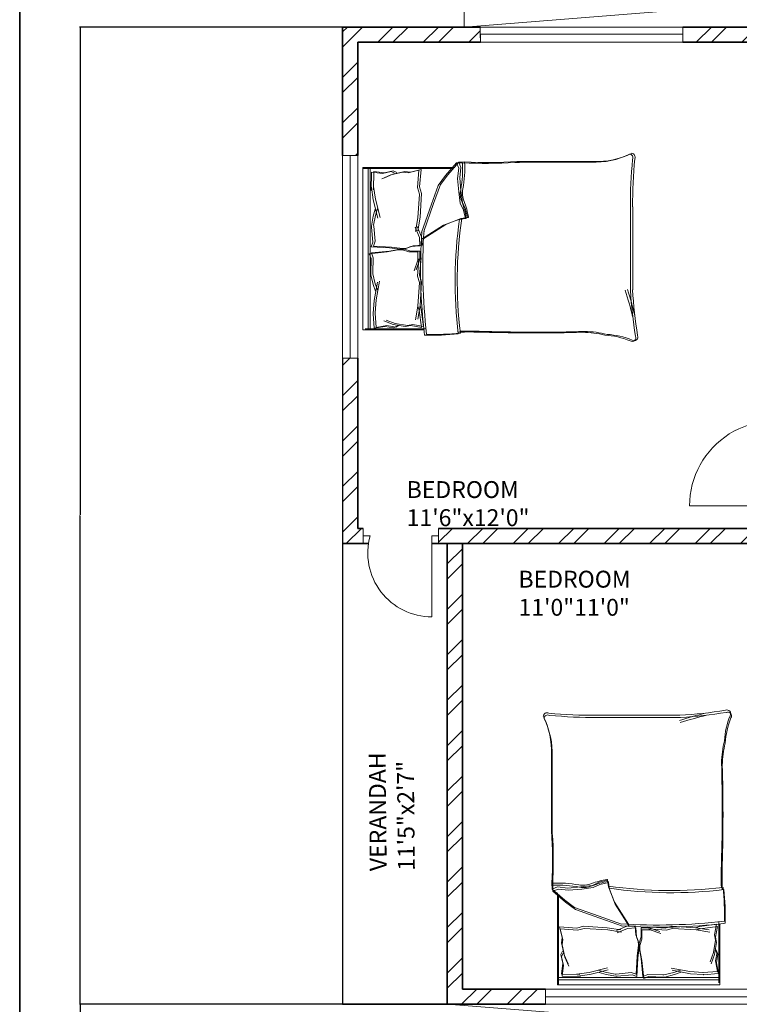
# Model space of a CAD drawing. Units: inches. Extents: x 1885 to 2748, y 783 to 2421.
# Tile 40 of 117: x 1885 to 2098, y 1558 to 1850. Entities that reach past the tile are written whole.
import ezdxf

# ---------------------------------------------------------------- set-up
doc = ezdxf.new("R2010")
doc.units = ezdxf.units.IN
for name, color, linetype, lineweight in [('A-ANNO-DIMS', 2, 'Continuous', 18), ('A-ANNO-TTLB', 7, 'Continuous', 35), ('A-AREA-IDEN', 7, 'Continuous', 18), ('A-DOOR', 31, 'Continuous', 18), ('A-FLOR-BALC', 7, 'Continuous', 25), ('A-FLOR-OPEN', 8, 'Continuous', 13), ('A-FURN', 8, 'Continuous', 13), ('A-GLAZ', 181, 'Continuous', 18), ('A-WALL', 7, 'Continuous', 35)]:
    doc.layers.add(name, color=color, linetype=linetype, lineweight=lineweight)
doc.layers.add('A-WALL-PATT', color=85, linetype='Continuous', lineweight=13, true_color=0x58ba48)
doc.styles.get("Standard").update_dxf_attribs({"font": 'arial.ttf'})
doc.dimstyles.get("Standard").update_dxf_attribs({"dimtxt": 0.18, "dimasz": 0.18, "dimexe": 0.18, "dimexo": 0.0625, "dimgap": 0.09, "dimtad": 0, "dimtih": 1, "dimtoh": 1, "dimdec": 4, "dimzin": 0, "dimdsep": 46, "dimtxsty": 'Standard', "dimcen": 0.09, "dimadec": 0, "dimazin": 0, "dimtfac": 1, "dimtdec": 4, "dimtofl": 0, "dimtmove": 0, "dimatfit": 3, "dimfxl": 1, "dimtolj": 1, "dimtzin": 0, "dimarcsym": 0})

# ---------------------------------------------------------------- blocks, each defined once
blk = doc.blocks.new('BED-DOUBLE')
for p, q in [((27.75, 52.87), (24.5, 49.16)), ((27.75, 52.87), (24.5, 49.16)), ((28.39, 53.09), (25.14, 49.39)), ((28.39, 53.09), (25.14, 49.39)), ((29.49, 52.95), (27.75, 52.87, 3.87)), ((29.49, 52.95), (27.75, 52.87, 3.87)), ((28.37, 51.33), (27.75, 52.87)), ((28.37, 51.33), (27.75, 52.87)), ((30.13, 53.17), (28.39, 53.09, 3.87)), ((30.13, 53.17), (28.39, 53.09, 3.87)), ((29.01, 51.56), (28.39, 53.09)), ((29.01, 51.56), (28.39, 53.09)), ((0, 51.49), (0.64, 51.49)), ((0, 3.47), (0, 51.49)), ((0, 51.26), (26.61, 51.26)), ((0, 51.26), (26.61, 51.26)), ((0.64, 51.49), (27.25, 51.49)), ((0.64, 51.49), (27.25, 51.49)), ((1.54, 3.47), (1.54, 51.26)), ((1.54, 3.47), (1.54, 51.26)), ((2.18, 3.7), (2.18, 51.49)), ((2.18, 3.7), (2.18, 51.49)), ((2.56, 50.11), (2.46, 44.71)), ((2.56, 50.11), (2.46, 44.71)), ((2.56, 50.11), (5.77, 49.73)), ((2.56, 50.11), (5.77, 49.73)), ((3.2, 50.34), (3.1, 44.94)), ((3.2, 50.34), (3.1, 44.94)), ((3.2, 50.34), (6.41, 49.96)), ((3.2, 50.34), (6.41, 49.96)), ((5.77, 49.73), (8.34, 50.33)), ((5.77, 49.73), (8.34, 50.33)), ((6.41, 49.96), (8.98, 50.56)), ((6.41, 49.96), (8.98, 50.56)), ((11.83, 50.11), (8.26, 49.31)), ((11.83, 50.11), (8.26, 49.31)), ((8.34, 50.33), (9.39, 49.81)), ((8.34, 50.33), (9.39, 49.81)), ((12.47, 50.34), (8.9, 49.54)), ((12.47, 50.34), (8.9, 49.54)), ((8.98, 50.56), (10.03, 50.04)), ((8.98, 50.56), (10.03, 50.04)), ((13.44, 49.92), (11.83, 50.11)), ((13.44, 49.92), (11.83, 50.11)), ((14.08, 50.15), (12.47, 50.34)), ((14.08, 50.15), (12.47, 50.34)), ((16.58, 50.7), (13.44, 49.92)), ((16.58, 50.7), (13.44, 49.92)), ((17.22, 50.93), (14.08, 50.15)), ((17.22, 50.93), (14.08, 50.15)), ((16.17, 45.57), (16.58, 50.7)), ((16.17, 45.56), (16.58, 50.7)), ((16.81, 45.79), (17.22, 50.93)), ((16.81, 45.79), (17.22, 50.93)), ((28.06, 48.23), (28.37, 51.33)), ((28.06, 48.23), (28.37, 51.33)), ((28.7, 48.46), (29.01, 51.56)), ((28.7, 48.46), (29.01, 51.56)), ((8.26, 49.31), (5.58, 48.13)), ((8.26, 49.31), (5.58, 48.13)), ((8.9, 49.54), (6.22, 48.36)), ((8.9, 49.54), (6.22, 48.36)), ((24.5, 49.16), (22.33, 46.22)), ((24.5, 49.16), (22.33, 46.22)), ((25.14, 49.39), (22.97, 46.45)), ((25.14, 49.39), (22.97, 46.45)), ((28.37, 44.36), (28.06, 48.23)), ((28.37, 44.36), (28.06, 48.23)), ((29.01, 44.59), (28.7, 48.46)), ((29.01, 44.59), (28.7, 48.46)), ((2.46, 44.71), (2.55, 45.71)), ((2.46, 44.71), (2.55, 45.71)), ((2.55, 45.71), (3.07, 41.91)), ((2.55, 45.71), (3.07, 41.91)), ((3.1, 44.94), (3.19, 45.94)), ((3.1, 44.94), (3.19, 45.94)), ((3.19, 45.94), (3.71, 42.14)), ((3.19, 45.94), (3.71, 42.14)), ((16.73, 43.6), (16.17, 45.57)), ((16.73, 43.6), (16.17, 45.56)), ((17.37, 43.83), (16.81, 45.79)), ((17.37, 43.83), (16.81, 45.79)), ((16.94, 36.82), (17.37, 43.83)), ((16.94, 36.82), (17.37, 43.83)), ((22.33, 46.22), (20.32, 40.64)), ((22.33, 46.22), (20.32, 40.64)), ((22.97, 46.45), (20.96, 40.87)), ((22.97, 46.45), (20.96, 40.87)), ((28.83, 40.95), (28.37, 44.36)), ((28.83, 40.95), (28.37, 44.36)), ((29.47, 41.18), (29.01, 44.59)), ((29.47, 41.18), (29.01, 44.59)), ((3.07, 41.91), (4.43, 36.49)), ((3.07, 41.91), (4.43, 36.49)), ((3.71, 42.14), (5.07, 36.72)), ((3.71, 42.14), (5.07, 36.72)), ((16.3, 36.59), (16.73, 43.6)), ((16.3, 36.59), (16.73, 43.6)), ((20.96, 40.87), (18.03, 32.53)), ((20.96, 40.87), (18.03, 32.53)), ((29.76, 38.94), (28.83, 40.95)), ((29.76, 38.94), (28.83, 40.95)), ((30.4, 39.17), (29.47, 41.18)), ((30.4, 39.17), (29.47, 41.18)), ((3.68, 39.2), (3.08, 37.13)), ((3.68, 39.2), (3.08, 37.13)), ((4.32, 39.43), (3.72, 37.36)), ((4.32, 39.43), (3.72, 37.36)), ((20.32, 40.64), (17.39, 32.3)), ((20.32, 40.64), (17.39, 32.3)), ((30.38, 36.46), (29.76, 38.94)), ((30.38, 36.46), (29.76, 38.94)), ((31.02, 36.69), (30.4, 39.17)), ((31.02, 36.69), (30.4, 39.17)), ((79.25, 15.06), (79.25, 39.68)), ((79.25, 15.06), (79.25, 39.68)), ((79.89, 15.29), (79.89, 39.9)), ((79.89, 15.29), (79.89, 39.9)), ((3.08, 37.13), (2.54, 34.2)), ((3.08, 37.13), (2.54, 34.2)), ((3.72, 37.36), (3.18, 34.43)), ((3.72, 37.36), (3.18, 34.43)), ((15.63, 32.56), (16.3, 36.59)), ((15.63, 32.56), (16.3, 36.59)), ((16.27, 32.79), (16.94, 36.82)), ((16.27, 32.79), (16.94, 36.82)), ((23.88, 34.45), (28.37, 36.15)), ((23.88, 34.45), (28.37, 36.15)), ((24.52, 34.68), (29.01, 36.38)), ((24.52, 34.68), (29.01, 36.38)), ((28.37, 36.15), (30.38, 36.46)), ((28.37, 36.15), (30.38, 36.46)), ((29.01, 36.38), (31.02, 36.69)), ((29.01, 36.38), (31.02, 36.69)), ((2.54, 34.2), (2.56, 33.88)), ((2.54, 34.2), (2.56, 33.88)), ((2.56, 33.88), (2.98, 29.45)), ((2.56, 33.88), (2.98, 29.45)), ((3.18, 34.43), (3.2, 34.11)), ((3.18, 34.43), (3.2, 34.11)), ((3.2, 34.11), (3.62, 29.68)), ((3.2, 34.11), (3.62, 29.68)), ((16.74, 30.75), (15.46, 33.82)), ((16.74, 30.75), (15.46, 33.82)), ((17.38, 30.98), (16.1, 34.05)), ((17.38, 30.98), (16.1, 34.05)), ((17.39, 30.26), (23.88, 34.45)), ((17.39, 30.26), (23.88, 34.45)), ((18.03, 30.49), (24.52, 34.68)), ((18.03, 30.49), (24.52, 34.68)), ((2.98, 29.45), (2.5, 27.98)), ((2.98, 29.45), (2.5, 27.98)), ((3.62, 29.68), (3.13, 28.2)), ((3.62, 29.68), (3.13, 28.2)), ((16.9, 28.3), (16.74, 30.75)), ((16.9, 28.3), (16.74, 30.75)), ((17.54, 28.52), (17.38, 30.98)), ((17.54, 28.52), (17.38, 30.98)), ((1.87, 25.98), (7.22, 26.56)), ((1.87, 25.98), (7.22, 26.56)), ((2.5, 27.98), (7.87, 27.73)), ((2.5, 27.98), (7.87, 27.73)), ((2.51, 26.21), (7.86, 26.79)), ((2.51, 26.21), (7.86, 26.79)), ((3.13, 28.2), (8.51, 27.96)), ((3.13, 28.2), (8.51, 27.96)), ((7.22, 26.56), (10.4, 27.14)), ((7.22, 26.56), (10.4, 27.14)), ((7.86, 26.79), (11.04, 27.37)), ((7.86, 26.79), (11.04, 27.37)), ((7.87, 27.73), (11.08, 27.35)), ((7.87, 27.73), (11.08, 27.35)), ((8.51, 27.96), (11.72, 27.58)), ((8.51, 27.96), (11.72, 27.58)), ((10.4, 27.14), (11.71, 27.14)), ((10.4, 27.14), (11.71, 27.14)), ((11.04, 27.37), (12.35, 27.37)), ((11.04, 27.37), (12.35, 27.37)), ((11.08, 27.35), (12.38, 27.43)), ((11.08, 27.35), (12.38, 27.43)), ((11.71, 27.14), (13.59, 26.56)), ((11.71, 27.14), (13.59, 26.56)), ((11.72, 27.58), (13.02, 27.66)), ((11.72, 27.58), (13.02, 27.66)), ((12.35, 27.37), (14.22, 26.79)), ((12.35, 27.37), (14.22, 26.79)), ((12.38, 27.43), (14.22, 28.13)), ((12.38, 27.43), (14.22, 28.13)), ((13.02, 27.66), (14.86, 28.36)), ((13.02, 27.66), (14.86, 28.36)), ((13.59, 26.56), (16.27, 26.56)), ((13.59, 26.56), (16.27, 26.56)), ((14.22, 28.13), (16.9, 28.3)), ((14.22, 28.13), (16.9, 28.3)), ((14.22, 26.79), (16.91, 26.79)), ((14.22, 26.79), (16.91, 26.79)), ((14.86, 28.36), (17.54, 28.52)), ((14.86, 28.36), (17.54, 28.52)), ((16.27, 26.56), (16.27, 24.1)), ((16.27, 26.56), (16.27, 24.1)), ((16.91, 26.79), (16.91, 24.33)), ((16.91, 26.79), (16.91, 24.33)), ((2.45, 24.54), (1.87, 25.98)), ((2.45, 24.54), (1.87, 25.98)), ((2.31, 20.09), (2.45, 24.54)), ((2.31, 20.09), (2.45, 24.54)), ((3.09, 24.76), (2.51, 26.21)), ((3.09, 24.76), (2.51, 26.21)), ((2.95, 20.32), (3.09, 24.76)), ((2.95, 20.32), (3.09, 24.76)), ((16.27, 24.1), (15.18, 20.96)), ((16.27, 24.1), (15.18, 20.96)), ((16.91, 24.33), (15.82, 21.19)), ((16.91, 24.33), (15.82, 21.19)), ((16.17, 19.38), (16.58, 24.51)), ((16.17, 19.38), (16.58, 24.51)), ((16.81, 19.61), (17.22, 24.74)), ((16.81, 19.61), (17.22, 24.74)), ((2.31, 19.77), (2.31, 20.09)), ((2.31, 19.77), (2.31, 20.09)), ((3.03, 16.88), (2.31, 19.77)), ((3.03, 16.88), (2.31, 19.77)), ((2.95, 20), (2.95, 20.32)), ((2.95, 20), (2.95, 20.32)), ((3.67, 17.11), (2.95, 20)), ((3.67, 17.11), (2.95, 20)), ((3.32, 12.11), (4.33, 17.6)), ((3.32, 12.11), (4.33, 17.6)), ((3.96, 12.34), (4.97, 17.83)), ((3.96, 12.34), (4.97, 17.83)), ((16.73, 17.42), (16.17, 19.38)), ((16.73, 17.42), (16.17, 19.38)), ((17.37, 17.65), (16.81, 19.61)), ((17.37, 17.65), (16.81, 19.61)), ((16.94, 10.64), (17.37, 17.65)), ((16.94, 10.64), (17.37, 17.65)), ((3.75, 14.85), (3.03, 16.88)), ((3.75, 14.85), (3.03, 16.88)), ((4.39, 15.08), (3.67, 17.11)), ((4.39, 15.08), (3.67, 17.11)), ((16.3, 10.41), (16.73, 17.42)), ((16.3, 10.41), (16.73, 17.42)), ((3.03, 8.28), (3.32, 12.11)), ((3.03, 8.28), (3.32, 12.11)), ((3.67, 8.51), (3.96, 12.34)), ((3.67, 8.51), (3.96, 12.34)), ((15.63, 6.38), (16.3, 10.41)), ((15.63, 6.38), (16.3, 10.41)), ((16.27, 6.61), (16.94, 10.64)), ((16.27, 6.61), (16.94, 10.64)), ((16.3, 10.41), (16.62, 9.28)), ((16.3, 10.41), (16.62, 9.28)), ((16.62, 9.28), (17.34, 4.18)), ((16.62, 9.28), (17.34, 4.18)), ((16.94, 10.64), (17.26, 9.51)), ((16.94, 10.64), (17.26, 9.51)), ((17.26, 9.51), (17.98, 4.41)), ((17.26, 9.51), (17.98, 4.41)), ((3.01, 8.18), (3.03, 8.28)), ((3.01, 8.18), (3.03, 8.28)), ((3.34, 3.9), (3.01, 8.18)), ((3.34, 3.9), (3.01, 8.18)), ((3.65, 8.41), (3.67, 8.51)), ((3.65, 8.41), (3.67, 8.51)), ((3.98, 4.13), (3.65, 8.41)), ((3.98, 4.13), (3.65, 8.41)), ((8.96, 5.05), (6.21, 6.06)), ((8.96, 5.05), (6.21, 6.06)), ((9.6, 5.28), (6.85, 6.29)), ((9.6, 5.28), (6.85, 6.29)), ((18.11, 3.47), (0, 3.47)), ((18.11, 3.47), (0, 3.47)), ((18.75, 3.7), (0.64, 3.7)), ((18.75, 3.7), (0.64, 3.7)), ((3.32, 3.89), (6.5, 4.47)), ((3.32, 3.89), (6.5, 4.47)), ((3.96, 4.12), (7.14, 4.7)), ((3.96, 4.12), (7.14, 4.7)), ((6.5, 4.47), (9.1, 4.04)), ((6.5, 4.47), (9.1, 4.04)), ((7.14, 4.7), (9.74, 4.27)), ((7.14, 4.7), (9.74, 4.27)), ((12.57, 4.47), (8.96, 5.05)), ((12.57, 4.47), (8.96, 5.05)), ((9.1, 4.04), (10.12, 4.62)), ((9.1, 4.04), (10.12, 4.62)), ((13.21, 4.7), (9.6, 5.28)), ((13.21, 4.7), (9.6, 5.28)), ((9.74, 4.27), (10.75, 4.84)), ((9.74, 4.27), (10.75, 4.84)), ((14.16, 4.76), (12.57, 4.47)), ((14.16, 4.76), (12.57, 4.47)), ((14.8, 4.99), (13.21, 4.7)), ((14.8, 4.99), (13.21, 4.7)), ((17.34, 4.18), (14.16, 4.76)), ((17.34, 4.18), (14.16, 4.76)), ((17.98, 4.41), (14.8, 4.99)), ((17.98, 4.41), (14.8, 4.99))]:
    blk.add_line(p, q)
for centre, radius, start, end in [((68.67, 76.16), 23.07, 267.4714, 296.4681), ((68.67, 76.16), 23.07, 267.4714, 296.4681), ((69.31, 76.38), 23.07, 267.4714, 296.4681), ((69.31, 76.38), 23.07, 267.4714, 296.4681), ((78.87, 54.41), 1.1, 332.6588, 86.02), ((78.87, 54.41), 1.1, 332.6588, 86.02), ((79.51, 54.64), 1.1, 332.6588, 86.02), ((79.51, 54.64), 1.1, 332.6588, 86.02), ((-6.65, 51.33), 36.18, 349.8763, 2.5657), ((-6.65, 51.33), 36.18, 349.8763, 2.5657), ((36.32, 182.26), 129.5, 266.9791, 273.8365), ((36.32, 182.26), 129.5, 266.9791, 273.8365), ((-6.01, 51.55), 36.18, 349.8763, 2.5657), ((-6.01, 51.55), 36.18, 349.8763, 2.5657), ((36.96, 182.49), 129.5, 266.9791, 273.8365), ((36.96, 182.49), 129.5, 266.9791, 273.8365), ((67.83, -4508.74), 4561.86, 90.00217, 90.28689), ((67.83, -4508.75), 4561.86, 90.00217, 90.28689), ((68.46, -4508.52), 4561.86, 90.00217, 90.28689), ((68.46, -4508.52), 4561.86, 90.00217, 90.28689), ((212.28, 41.15), 133.04, 174.4998, 180.6351), ((212.28, 41.15), 133.04, 174.4998, 180.6351), ((212.92, 41.38), 133.04, 174.4998, 180.6351), ((212.92, 41.38), 133.04, 174.4998, 180.6351), ((35.07, 43.74), 6.22, 168.6608, 203.7384), ((35.07, 43.74), 6.22, 168.6608, 203.7384), ((35.71, 43.97), 6.22, 168.6608, 203.7384), ((35.71, 43.97), 6.22, 168.6608, 203.7384), ((1.49, 31.15), 29.65, 10.6617, 19.8806), ((1.49, 31.15), 29.65, 10.6617, 19.8806), ((2.13, 31.38), 29.65, 10.6617, 19.8806), ((2.13, 31.38), 29.65, 10.6617, 19.8806), ((156.32, 17.75), 129.02, 171.7845, 186.9006), ((156.32, 17.75), 129.02, 171.7845, 186.9006), ((156.96, 17.98), 129.02, 171.7845, 186.9006), ((156.96, 17.98), 129.02, 171.7845, 186.9006), ((30.44, 36.64), 0.185, 250.2464, 1.1377), ((30.44, 36.63), 0.185, 250.2464, 1.1377), ((31.08, 36.86), 0.185, 250.2464, 1.1377), ((31.08, 36.86), 0.185, 250.2464, 1.1377), ((182.06, 21.36), 164.97, 176.0865, 186.7821), ((182.06, 21.36), 164.97, 176.0865, 186.7821), ((182.7, 21.59), 164.97, 176.0865, 186.7821), ((182.7, 21.59), 164.97, 176.0865, 186.7821), ((-23.71, -17.22), 106.46, 13.3832, 17.7053), ((-23.71, -17.22), 106.46, 13.3832, 17.7053), ((-23.07, -16.99), 106.46, 13.3832, 17.7053), ((-23.07, -16.99), 106.46, 13.3832, 17.7053), ((200.84, 21.43), 121.76, 182.9958, 189.4091), ((200.84, 21.43), 121.76, 182.9958, 189.4091), ((201.48, 21.65), 121.76, 182.9958, 189.4091), ((201.48, 21.65), 121.76, 182.9958, 189.4091), ((31.82, -167.08), 170.11, 88.4762, 91.0082), ((31.82, -167.08), 170.11, 88.4762, 91.0082), ((51.26, 485.05), 482.31, 268.2277, 271.7185), ((51.26, 485.05), 482.31, 268.2277, 271.7185), ((65.16, -26.67), 29.63, 76.0648, 88.9113), ((65.16, -26.67), 29.63, 76.0648, 88.9113), ((20.1, 85.16), 83.31, 268.7218, 275.604), ((20.1, 85.16), 83.31, 268.7218, 275.604), ((20.74, 85.39), 83.31, 268.7218, 275.604), ((20.74, 85.39), 83.31, 268.7218, 275.604), ((31.18, -167.31), 170.11, 88.4762, 91.0082), ((31.18, -167.31), 170.11, 88.4762, 91.0082), ((50.62, 484.82), 482.31, 268.2277, 271.7185), ((50.62, 484.82), 482.31, 268.2277, 271.7185), ((64.52, -26.9), 29.63, 76.0648, 88.9113), ((64.52, -26.9), 29.63, 76.0648, 88.9113), ((70.28, -21.66), 23.56, 67.9751, 86.652), ((70.28, -21.66), 23.56, 67.9751, 86.652), ((70.92, -21.43), 23.56, 67.9751, 86.652), ((70.92, -21.43), 23.56, 67.9751, 86.652), ((79.72, 1.09), 1.09, 236.1736, 23.4781), ((79.72, 1.09), 1.09, 236.1736, 23.4781), ((80.36, 1.31), 1.09, 236.1736, 23.4781), ((80.36, 1.31), 1.09, 236.1736, 23.4781)]:
    blk.add_arc(centre, radius, start, end)
blk = doc.blocks.new('WIN-60')
for p, q in [((0, 60), (4.5, 60)), ((0, 60), (0, 0)), ((4.5, 60), (2.25, 60)), ((2.25, 60), (2.25, 0)), ((4.5, 0), (4.5, 60)), ((2.25, 0), (0, 0)), ((0, 0), (4.5, 0))]:
    blk.add_line(p, q)
blk = doc.blocks.new('*D46')
at = {"layer": 'A-ANNO-DIMS', "color": 0, "lineweight": -2, "transparency": 16777216}
for p, q in [((1980.71, 1558.01), (1902.84, 1558.01)), ((1903.02, 1557.83), (1903.02, 1541.19)), ((1903.02, 1524.19), (1903.02, 1540.82)), ((1980.71, 1524.01), (1902.84, 1524.01))]:
    blk.add_line(p, q, dxfattribs=at)
at = {"layer": 'A-ANNO-DIMS', "color": 0, "transparency": 16777216}
for points in [[(1902.99, 1557.83), (1903.05, 1557.83), (1903.02, 1558.01)], [(1902.99, 1524.19), (1903.05, 1524.19), (1903.02, 1524.01)]]:
    blk.add_solid(points, dxfattribs=at)
at = {"layer": 'Defpoints', "color": 0, "transparency": 16777216}
for p in [(1903.02, 1558.01), (1980.77, 1558.01), (1980.77, 1524.01)]:
    blk.add_point(p, dxfattribs=at)
at = {"layer": 'A-ANNO-DIMS', "color": 0, "transparency": 16777216, "insert": (1903.02, 1541.01), "char_height": 0.18, "attachment_point": 5}
blk.add_mtext('\\A1;34', dxfattribs=at)
blk = doc.blocks.new('*D47')
at = {"layer": 'A-ANNO-DIMS', "color": 0, "lineweight": -2, "transparency": 16777216}
for p, q in [((1980.71, 1847.51), (1902.84, 1847.51)), ((1903.02, 1847.33), (1903.02, 1702.94)), ((1903.02, 1558.19), (1903.02, 1702.57)), ((1980.71, 1558.01), (1902.84, 1558.01))]:
    blk.add_line(p, q, dxfattribs=at)
at = {"layer": 'A-ANNO-DIMS', "color": 0, "transparency": 16777216}
for points in [[(1902.99, 1847.33), (1903.05, 1847.33), (1903.02, 1847.51)], [(1902.99, 1558.19), (1903.05, 1558.19), (1903.02, 1558.01)]]:
    blk.add_solid(points, dxfattribs=at)
at = {"layer": 'Defpoints', "color": 0, "transparency": 16777216}
for p in [(1903.02, 1847.51), (1980.77, 1847.51), (1980.77, 1558.01)]:
    blk.add_point(p, dxfattribs=at)
at = {"layer": 'A-ANNO-DIMS', "color": 0, "transparency": 16777216, "insert": (1903.02, 1702.76), "char_height": 0.18, "attachment_point": 5}
blk.add_mtext('\\A1;289.5', dxfattribs=at)

msp = doc.modelspace()

# ---------------------------------------------------------------- hatches: boundary and pattern name
at = {"layer": 'A-WALL-PATT'}
h = msp.add_hatch(dxfattribs=at)
h.set_pattern_fill('ANSI32', color=256)
h.paths.add_polyline_path([(2007.77, 2318.01), (1980.77, 2318.01), (1980.77, 2281.22), (1985.27, 2281.22), (1985.27, 2313.51), (2007.77, 2313.51), (2007.77, 2315.76)])
h.paths.add_polyline_path([(2094.32, 2318.01), (2067.77, 2318.01), (2067.77, 2313.51), (2094.32, 2313.51), (2094.32, 2315.76)])
h.paths.add_polyline_path([(2131.37, 2315.76), (2131.37, 2318.01), (2131.19, 2318.01), (2112.61, 2318.01), (2112.61, 2313.51), (2117.27, 2313.51), (2117.27, 2255.2), (2121.77, 2255.2), (2121.77, 2313.51), (2131.37, 2313.51)])
h.paths.add_polyline_path([(2190.51, 2318.01), (2155.37, 2318.01), (2155.37, 2313.51), (2169.77, 2313.51), (2169.77, 2229.51), (2121.77, 2229.51), (2121.77, 2233.45), (2119.52, 2233.45), (2117.27, 2233.45), (2117.27, 2201.1), (2121.77, 2201.1), (2121.77, 2225.01), (2169.77, 2225.01), (2169.77, 2165.01), (2306.27, 2165.01), (2306.27, 2066.01), (2310.77, 2066.01), (2344.27, 2066.01), (2486.27, 2066.01), (2486.27, 1886.01), (2483.02, 1886.01), (2483.02, 1881.51), (2486.27, 1881.51), (2486.27, 1880.68), (2490.77, 1880.68), (2490.77, 2070.51), (2344.27, 2070.51), (2310.77, 2070.51), (2310.77, 2165.01), (2310.77, 2173.64), (2308.52, 2173.64), (2306.27, 2173.64), (2306.27, 2169.51), (2174.27, 2169.51), (2174.27, 2313.51), (2190.51, 2313.51), (2190.51, 2315.76)])
h.paths.add_polyline_path([(1985.27, 2221.22), (1980.77, 2221.22), (1980.77, 2165.01), (1992.77, 2165.01), (1992.77, 2141.93), (1997.27, 2141.93), (1997.27, 2165.01), (2117.27, 2165.01), (2117.27, 2163.13), (2121.77, 2163.13), (2121.77, 2172.73), (2119.52, 2172.73), (2117.27, 2172.73), (2117.27, 2169.51), (1985.27, 2169.51)])
h.paths.add_polyline_path([(1997.27, 2105.93), (1992.77, 2105.93), (1992.77, 2070.51), (2016.77, 2070.51), (2016.77, 2059.12), (2019.02, 2059.12), (2021.27, 2059.12), (2021.27, 2070.51), (2117.27, 2070.51), (2117.27, 2022.51), (2114.42, 2022.51), (2114.42, 2018.01), (2123.63, 2018.01), (2123.63, 2020.26), (2123.63, 2022.51), (2121.77, 2022.51), (2121.77, 2142.59), (2119.52, 2142.59), (2117.27, 2142.59), (2117.27, 2075.01), (1997.27, 2075.01)])
h.paths.add_polyline_path([(2092.03, 2020.26), (2092.03, 2022.51), (2021.27, 2022.51), (2021.27, 2035.12), (2016.77, 2035.12), (2016.77, 2018.01), (2016.77, 1978.78), (2021.27, 1978.78), (2021.27, 2018.01), (2092.03, 2018.01)])
h.paths.add_polyline_path([(2260.94, 2022.51), (2153.1, 2022.51), (2153.1, 2020.26), (2153.1, 2018.01), (2155.27, 2018.01), (2155.27, 1886.01), (2107.63, 1886.01), (2107.63, 1881.51), (2182.91, 1881.51), (2182.91, 1883.76), (2182.91, 1886.01), (2159.77, 1886.01), (2159.77, 2018.01), (2260.94, 2018.01), (2260.94, 2020.26)])
h.paths.add_polyline_path([(2047.63, 1883.76), (2047.63, 1886.01), (2021.27, 1886.01), (2021.27, 1918.78), (2019.02, 1918.78), (2016.77, 1918.78), (2016.77, 1881.51), (2047.63, 1881.51)])
h.paths.add_polyline_path([(2306.36, 1883.76), (2306.36, 1886.01), (2296.27, 1886.01), (2296.27, 1982.01), (2316.54, 1982.01), (2316.54, 1984.26), (2316.54, 1986.51), (2296.27, 1986.51), (2296.27, 2022.51), (2289.28, 2022.51), (2289.28, 2018.01), (2291.77, 2018.01), (2291.77, 1886.01), (2242.91, 1886.01), (2242.91, 1881.51), (2306.36, 1881.51)], flags=17)
h.paths.add_polyline_path([(1985.27, 1843.01), (2021.6, 1843.01), (2021.53, 1845.44), (2021.48, 1847.51), (1980.77, 1847.51), (1980.77, 1809.45), (1985.27, 1809.45)])
h.paths.add_polyline_path([(2131.48, 1845.26), (2131.48, 1847.51), (2081.53, 1847.51), (2081.53, 1843.01), (2117.27, 1843.01), (2117.27, 1784.15), (2119.52, 1784.15), (2121.77, 1784.15), (2121.77, 1843.01), (2131.48, 1843.01)])
h.paths.add_polyline_path([(2203.89, 1847.51), (2155.48, 1847.51), (2155.48, 1843.01), (2169.77, 1843.01), (2169.77, 1759.01), (2121.77, 1759.01), (2121.77, 1761.46), (2117.27, 1761.46), (2117.27, 1730.43), (2121.77, 1730.43), (2121.77, 1754.51), (2177.42, 1754.51), (2177.42, 1756.76), (2177.42, 1759.01), (2174.27, 1759.01), (2174.27, 1843.01), (2203.89, 1843.01)])
h.paths.add_polyline_path([(2335.55, 1845.26), (2335.55, 1847.51), (2239.89, 1847.51), (2239.89, 1843.01), (2306.27, 1843.01), (2306.27, 1759.01), (2199.49, 1759.01), (2199.49, 1754.51), (2310.77, 1754.51), (2310.77, 1843.01), (2335.55, 1843.01)])
h.paths.add_polyline_path([(2348.77, 2022.51), (2344.27, 2022.51), (2344.27, 1986.51), (2341.68, 1986.51), (2341.68, 1982.01), (2344.27, 1982.01), (2344.27, 1886.01), (2330.36, 1886.01), (2330.36, 1881.51), (2361.63, 1881.51), (2361.63, 1883.76), (2361.63, 1886.01), (2348.77, 1886.01)], flags=17)
h.paths.add_polyline_path([(2283.25, 2315.76), (2283.25, 2318.01), (2238.51, 2318.01), (2238.51, 2313.51), (2283.25, 2313.51)], flags=17)
h.paths.add_polyline_path([(2363.27, 2348.01), (2388.68, 2348.01), (2388.68, 2350.26), (2388.68, 2352.51), (2358.77, 2352.51), (2358.77, 2348.01), (2358.77, 2318.01), (2344.48, 2318.01), (2344.48, 2313.51), (2358.77, 2313.51), (2358.77, 2229.51), (2310.77, 2229.51), (2310.77, 2231.95), (2306.27, 2231.95), (2306.27, 2205.61), (2310.77, 2205.61), (2310.77, 2225.01), (2358.77, 2225.01), (2358.77, 2211.51), (2452.33, 2211.51), (2452.33, 2213.76), (2452.33, 2216.01), (2363.27, 2216.01), (2363.27, 2318.01)])
h.paths.add_polyline_path([(2310.77, 2313.51), (2320.48, 2313.51), (2320.48, 2315.76), (2320.48, 2318.01), (2302.73, 2318.01), (2302.73, 2313.51), (2306.27, 2313.51), (2306.27, 2251.08), (2310.77, 2251.08)], flags=17)
h.paths.add_polyline_path([(2490.77, 2352.51), (2486.27, 2352.51), (2448.68, 2352.51), (2448.68, 2348.01), (2486.27, 2348.01), (2486.27, 2318.01), (2486.27, 2216.01), (2481.78, 2216.01), (2481.78, 2211.51), (2486.27, 2211.51), (2486.27, 2165.01), (2493.29, 2165.01), (2493.29, 2167.26), (2493.29, 2169.51), (2490.77, 2169.51), (2490.77, 2313.51), (2494.43, 2313.51), (2494.43, 2318.01), (2490.77, 2318.01)])
h.paths.add_polyline_path([(2534.65, 2318.01), (2515.69, 2318.01), (2515.69, 2313.51), (2534.65, 2313.51), (2534.65, 2315.76)])
h.paths.add_polyline_path([(2618.27, 2318.01), (2594.65, 2318.01), (2594.65, 2313.51), (2613.77, 2313.51), (2613.77, 2281.71), (2618.27, 2281.71)])
h.paths.add_polyline_path([(2618.27, 2221.71), (2613.77, 2221.71), (2613.77, 2169.51), (2554.02, 2169.51), (2554.02, 2165.01), (2613.77, 2165.01), (2613.77, 2152.88), (2618.27, 2152.88)])
h.paths.add_polyline_path([(2618.27, 2128.88), (2616.02, 2128.88), (2613.77, 2128.88), (2613.77, 2117.01), (2529.77, 2117.01), (2529.77, 2165.01), (2532.85, 2165.01), (2532.85, 2169.51), (2522.87, 2169.51), (2522.87, 2165.01), (2525.27, 2165.01), (2525.27, 2117.01), (2525.27, 2112.51), (2525.27, 2108.58), (2529.77, 2108.58), (2529.77, 2112.51), (2613.77, 2112.51), (2613.77, 2080.19), (2618.27, 2080.19)])
h.paths.add_polyline_path([(2618.27, 2044.19), (2616.02, 2044.19), (2613.77, 2044.19), (2613.77, 2015.51), (2529.77, 2015.51), (2529.77, 2088.58), (2527.52, 2088.58), (2525.27, 2088.58), (2525.27, 2011.01), (2613.77, 2011.01), (2613.77, 1956.75), (2618.27, 1956.75)])
h.paths.add_polyline_path([(2618.27, 1881.51), (2618.27, 1896.75), (2613.77, 1896.75), (2613.77, 1881.51), (2613.77, 1847.51), (2592.71, 1847.51), (2592.71, 1843.01), (2613.77, 1843.01), (2613.77, 1765.01), (2613.77, 1760.51), (2609.62, 1760.51), (2609.62, 1756.01), (2613.77, 1756.01), (2613.77, 1660.01), (2608.54, 1660.01), (2608.54, 1655.51), (2613.77, 1655.51), (2613.77, 1508.16), (2618.27, 1508.16)])
h.paths.add_polyline_path([(2565.77, 1843.01), (2569, 1843.01), (2569, 1847.51), (2490.77, 1847.51), (2490.77, 1849.7), (2488.52, 1849.7), (2486.27, 1849.7), (2486.27, 1847.51), (2477.27, 1847.51), (2477.27, 1838.51), (2477.27, 1821.49), (2486.27, 1821.49), (2486.27, 1838.51), (2561.27, 1838.51), (2561.27, 1765.01), (2486.27, 1765.01), (2486.27, 1786.16), (2477.27, 1786.16), (2477.27, 1765.01), (2477.27, 1756.01), (2486.27, 1756.01), (2565.77, 1756.01), (2585.62, 1756.01), (2585.62, 1758.26), (2585.62, 1760.51), (2565.77, 1760.51), (2565.77, 1765.01)])
h.paths.add_polyline_path([(2486.27, 1651.01), (2561.27, 1651.01), (2561.27, 1567.01), (2486.27, 1567.01), (2486.27, 1591.32), (2477.27, 1591.32), (2477.27, 1567.01), (2477.27, 1558.01), (2477.27, 1555.44), (2481.77, 1555.44), (2481.77, 1558.01), (2568.65, 1558.01), (2568.65, 1560.26), (2568.65, 1562.51), (2565.77, 1562.51), (2565.77, 1655.51), (2584.54, 1655.51), (2584.54, 1657.76), (2584.54, 1660.01), (2565.77, 1660.01), (2486.27, 1660.01), (2477.27, 1660.01), (2477.27, 1651.01), (2477.27, 1632.99), (2486.27, 1632.99)])
h.paths.add_polyline_path([(2449.97, 1883.76), (2449.97, 1886.01), (2421.63, 1886.01), (2421.63, 1881.51), (2449.97, 1881.51)], flags=17)
h.paths.add_polyline_path([(2447.27, 1847.51), (2395.55, 1847.51), (2395.55, 1843.01), (2442.77, 1843.01), (2442.77, 1809.27), (2447.27, 1809.27)])
h.paths.add_polyline_path([(1985.27, 1749.45), (1980.77, 1749.45), (1980.77, 1694.5), (1985.27, 1694.5), (1985.27, 1694.51), (1986.9, 1694.51), (1986.9, 1697.78), (1986.9, 1699.01), (1985.27, 1699.01)])
h.paths.add_polyline_path([(2152.77, 1699.01), (2121.77, 1699.01), (2121.77, 1703.67), (2119.52, 1703.67), (2117.27, 1703.67), (2117.27, 1699.01), (2009.22, 1699.01), (2009.22, 1694.51), (2148.27, 1694.51), (2148.27, 1692.63), (2152.77, 1692.63)])
h.paths.add_polyline_path([(2016.27, 1694.51), (2011.77, 1694.51), (2011.77, 1558.01), (2040.81, 1558.01), (2040.81, 1560.26), (2040.81, 1562.51), (2016.27, 1562.51)])
h.paths.add_polyline_path([(2152.77, 1663.02), (2150.52, 1663.02), (2148.27, 1663.02), (2148.27, 1562.51), (2100.81, 1562.51), (2100.81, 1558.01), (2165.12, 1558.01), (2165.12, 1560.26), (2165.12, 1562.51), (2152.77, 1562.51), (2152.77, 1610.51), (2224.77, 1610.51), (2224.77, 1607.99), (2229.27, 1607.99), (2229.27, 1615.01), (2152.77, 1615.01)])
h.paths.add_polyline_path([(2238.61, 1560.26), (2238.61, 1562.51), (2229.27, 1562.51), (2229.27, 1588.76), (2227.02, 1588.76), (2224.77, 1588.77), (2224.77, 1562.51), (2189.12, 1562.51), (2189.12, 1558.01), (2238.61, 1558.01)])
h.paths.add_polyline_path([(2336.02, 1560.26), (2336.02, 1562.51), (2310.77, 1562.51), (2310.77, 1656.35), (2308.52, 1656.35), (2306.27, 1656.35), (2306.27, 1562.51), (2286.61, 1562.51), (2286.61, 1558.01), (2336.02, 1558.01)])
h.paths.add_polyline_path([(2447.27, 1690.97), (2445.02, 1690.97), (2442.77, 1690.97), (2442.77, 1687.01), (2306.27, 1687.01), (2306.27, 1680.75), (2310.77, 1680.75), (2310.77, 1682.51), (2442.77, 1682.51), (2442.77, 1562.51), (2396.02, 1562.51), (2396.02, 1558.01), (2447.27, 1558.01)])
h.paths.add_polyline_path([(2447.27, 1749.27), (2445.02, 1749.27), (2442.77, 1749.27), (2442.77, 1717.23), (2447.27, 1717.23)])
h.paths.add_polyline_path([(2044.67, 1521.76), (2044.67, 1524.01), (2007.27, 1524.01), (2007.27, 1503.49), (2009.52, 1503.49), (2011.77, 1503.49), (2011.77, 1519.51), (2044.67, 1519.51)])
h.paths.add_polyline_path([(2177.97, 1521.76), (2177.97, 1524.01), (2104.67, 1524.01), (2104.67, 1519.51), (2145.77, 1519.51), (2145.77, 1387.51), (2143.37, 1387.51), (2143.37, 1383.01), (2251.59, 1383.01), (2251.59, 1385.26), (2251.59, 1387.51), (2150.27, 1387.51), (2150.27, 1519.51), (2177.97, 1519.51)])
h.paths.add_polyline_path([(2298.7, 1524.01), (2237.97, 1524.01), (2237.97, 1519.51), (2282.27, 1519.51), (2282.27, 1387.51), (2279.68, 1387.51), (2279.68, 1383.01), (2286.77, 1383.01), (2286.77, 1419.01), (2312.45, 1419.01), (2312.45, 1421.26), (2312.45, 1423.51), (2286.77, 1423.51), (2286.77, 1519.51), (2298.7, 1519.51), (2298.7, 1521.72)], flags=17)
h.paths.add_polyline_path([(2361.9, 1521.76), (2361.9, 1524.01), (2322.7, 1524.01), (2322.7, 1519.51), (2334.77, 1519.51), (2334.77, 1423.51), (2331.93, 1423.51), (2331.93, 1419.01), (2334.77, 1419.01), (2334.77, 1387.51), (2334.77, 1383.23), (2339.27, 1383.23), (2339.27, 1387.51), (2339.27, 1519.51), (2361.9, 1519.51)], flags=17)
h.paths.add_polyline_path([(2447.27, 1521.76), (2447.27, 1524.01), (2421.9, 1524.01), (2421.9, 1519.51), (2447.27, 1519.51)], flags=17)
h.paths.add_polyline_path([(2481.77, 1529.6), (2479.52, 1529.6), (2477.27, 1529.6), (2477.27, 1524.01), (2474.49, 1524.01), (2474.49, 1519.51), (2477.27, 1519.51), (2477.27, 1334.51), (2296.77, 1334.51), (2296.77, 1240.51), (2160.27, 1240.51), (2160.27, 1180.51), (2112.27, 1180.51), (2112.27, 1207.69), (2110.02, 1207.69), (2107.77, 1207.69), (2107.77, 1171.61), (2112.27, 1171.61), (2112.27, 1176.01), (2160.27, 1176.01), (2160.27, 1092.01), (2144.22, 1092.01), (2144.22, 1087.51), (2189.5, 1087.51), (2189.5, 1089.76), (2189.5, 1092.01), (2164.77, 1092.01), (2164.77, 1236.01), (2296.77, 1236.01), (2296.77, 1231.91), (2301.27, 1231.91), (2301.27, 1330.01), (2481.77, 1330.01), (2481.77, 1387.51)])
h.paths.add_polyline_path([(2618.27, 1448.16), (2613.77, 1448.16), (2613.77, 1382.51), (2529.77, 1382.51), (2525.27, 1382.51), (2525.27, 1307.06), (2529.77, 1307.06), (2529.77, 1378.01), (2613.77, 1378.01), (2613.77, 1354.99), (2618.27, 1354.99)])
h.paths.add_polyline_path([(2618.27, 1318.99), (2613.77, 1318.99), (2613.77, 1281.01), (2529.77, 1281.01), (2529.77, 1283.79), (2527.52, 1283.79), (2525.27, 1283.79), (2525.27, 1228.51), (2516.79, 1228.51), (2516.79, 1224.01), (2533.48, 1224.01), (2533.48, 1226.26), (2533.48, 1228.51), (2529.77, 1228.51), (2529.77, 1276.51), (2613.77, 1276.51), (2613.77, 1266.02), (2618.27, 1266.02)])
h.paths.add_polyline_path([(2618.27, 1134.96), (2613.77, 1134.96), (2613.77, 1092.01), (2594.54, 1092.01), (2594.54, 1087.51), (2618.27, 1087.51)])
h.paths.add_polyline_path([(2534.54, 1092.01), (2509.77, 1092.01), (2509.77, 1087.51), (2534.54, 1087.51), (2534.54, 1089.76)])
h.paths.add_polyline_path([(2481.27, 1224.01), (2484.12, 1224.01), (2484.12, 1226.26), (2484.12, 1228.51), (2476.77, 1228.51), (2476.77, 1198.51), (2471.61, 1198.51), (2471.61, 1194.01), (2476.77, 1194.01), (2476.77, 1062.01), (2436.89, 1062.01), (2436.89, 1057.51), (2476.77, 1057.51), (2481.27, 1057.51), (2481.27, 1062.01), (2481.27, 1087.51), (2485.35, 1087.51), (2485.35, 1089.76), (2485.35, 1092.01), (2481.27, 1092.01), (2481.27, 1117.51)])
h.paths.add_polyline_path([(2439.9, 1198.51), (2349.27, 1198.51), (2349.27, 1194.01), (2349.27, 1180.51), (2301.27, 1180.51), (2301.27, 1201.9), (2299.02, 1201.9), (2296.77, 1201.9), (2296.77, 1172.34), (2299.02, 1172.34), (2301.27, 1172.34), (2301.27, 1176.01), (2349.27, 1176.01), (2349.27, 1092.01), (2334.45, 1092.01), (2334.45, 1087.51), (2349.27, 1087.51), (2349.27, 1057.51), (2353.77, 1057.51), (2376.89, 1057.51), (2376.89, 1059.76), (2376.89, 1062.01), (2353.77, 1062.01), (2353.77, 1087.51), (2353.77, 1180.51), (2353.77, 1194.01), (2439.9, 1194.01), (2439.9, 1196.26)])
h.paths.add_polyline_path([(2270.6, 1089.76), (2270.6, 1092.01), (2249.5, 1092.01), (2249.5, 1087.51), (2270.6, 1087.51)], flags=17)
h.paths.add_polyline_path([(2310.45, 1092.01), (2301.27, 1092.01), (2301.27, 1153.29), (2296.77, 1153.29), (2296.77, 1092.01), (2293.79, 1092.01), (2293.79, 1087.51), (2310.45, 1087.51), (2310.45, 1089.76)], flags=17)
h.paths.add_polyline_path([(2112.27, 1150.33), (2110.02, 1150.33), (2107.77, 1150.33), (2107.77, 1092.01), (2104.47, 1092.01), (2104.47, 1087.51), (2120.22, 1087.51), (2120.22, 1089.76), (2120.22, 1092.01), (2112.27, 1092.01)])
h.paths.add_polyline_path([(2082.17, 1092.01), (2058.14, 1092.01), (2058.14, 1087.51), (2082.17, 1087.51), (2082.17, 1089.76)])
h.paths.add_polyline_path([(1975.77, 1145.64), (1971.27, 1145.64), (1971.27, 1087.51), (1980.77, 1087.51), (1998.14, 1087.51), (1998.14, 1089.76), (1998.14, 1092.01), (1985.27, 1092.01), (1975.77, 1092.01)])
h.paths.add_polyline_path([(2112.27, 1244.38), (2110.02, 1244.38), (2107.77, 1244.38), (2107.77, 1240.51), (1992.27, 1240.51), (1992.27, 1271.01), (1987.77, 1271.01), (1987.77, 1240.51), (1980.77, 1240.51), (1975.77, 1240.51), (1971.27, 1240.51), (1971.27, 1205.64), (1975.77, 1205.64), (1975.77, 1236.01), (2107.77, 1236.01), (2107.77, 1233.44), (2112.27, 1233.44), (2112.27, 1236.01)])
h.paths.add_polyline_path([(2112.27, 1383.01), (2114.78, 1383.01), (2114.78, 1385.26), (2114.78, 1387.51), (2102.48, 1387.51), (2102.48, 1383.01), (2107.77, 1383.01), (2107.77, 1335.01), (2011.77, 1335.01), (2011.77, 1349.94), (2007.27, 1349.94), (2007.27, 1335.01), (1987.77, 1335.01), (1987.77, 1330.51), (1987.77, 1307.01), (1992.27, 1307.01), (1992.27, 1330.51), (2007.27, 1330.51), (2107.77, 1330.51), (2107.77, 1264.71), (2112.27, 1264.71)])
h.paths.add_polyline_path([(2077.86, 1387.51), (2011.77, 1387.51), (2011.77, 1390.04), (2009.52, 1390.04), (2007.27, 1390.04), (2007.27, 1373.94), (2011.77, 1373.94), (2011.77, 1383.01), (2077.86, 1383.01)])
h.paths.add_polyline_path([(2011.77, 1443.49), (2007.27, 1443.49), (2007.27, 1410.25), (2011.77, 1410.25)])

# ---------------------------------------------------------------- linework, layer by layer
at = {"layer": 'A-ANNO-TTLB'}
msp.add_lwpolyline([(1885.16, 2409.17), (2748.2, 2409.17), (2748.2, 922.58), (1885.16, 922.58)], close=True, dxfattribs=at)
at = {"layer": 'A-DOOR'}
for p, q in [((2119.52, 1705.67), (2083.52, 1705.67)), ((1986.9, 1699.01), (1986.9, 1694.51)), ((1986.9, 1694.51), (1986.9, 1697.78)), ((1986.9, 1697.78), (1986.9, 1696.76)), ((2009.22, 1699.01), (2009.22, 1694.51)), ((1986.9, 1696.76), (1988.9, 1696.76)), ((2009.22, 1696.76), (2007.22, 1696.76)), ((2007.22, 1696.76), (2007.22, 1672.76)), ((2009.22, 1694.51), (2009.22, 1696.76))]:
    msp.add_line(p, q, dxfattribs=at)
for centre, radius, start, end in [((2108.72, 1705.67), 25.19, 64.6047, 180), ((2007.22, 1691.75), 18.99, 164.7185, 270)]:
    msp.add_arc(centre, radius, start, end, dxfattribs=at)
at = {"layer": 'A-FLOR-BALC'}
msp.add_line((1980.77, 1749.45), (1980.77, 1558.01), dxfattribs=at)
at = {"layer": 'A-FLOR-OPEN'}
for p, q in [((2016.77, 1881.51), (2016.77, 1847.51)), ((2016.77, 1847.51), (2447.27, 1881.51)), ((2447.27, 1524.01), (2011.77, 1558.01))]:
    msp.add_line(p, q, dxfattribs=at)
at = {"layer": 'A-GLAZ'}
for p, q in [((2021.48, 1847.51), (2021.6, 1843.01)), ((2081.53, 1847.51), (2021.48, 1847.51)), ((2081.53, 1845.44), (2081.53, 1847.51)), ((2081.53, 1847.51), (2081.53, 1843.01)), ((2021.6, 1843.01), (2021.53, 1845.44)), ((2021.53, 1845.44), (2081.53, 1845.44)), ((2021.6, 1843.01), (2081.53, 1843.01))]:
    msp.add_line(p, q, dxfattribs=at)
at = {"layer": 'A-WALL'}
for p, q in [((1980.77, 1847.51), (2021.48, 1847.51)), ((1980.77, 1847.51), (1980.77, 1809.45)), ((2081.53, 1847.51), (2131.48, 1847.51)), ((1985.27, 1843.01), (2021.6, 1843.01)), ((1985.27, 1843.01), (1985.27, 1809.45)), ((2081.53, 1843.01), (2117.27, 1843.01)), ((1985.27, 1749.45), (1985.27, 1699.01)), ((1985.27, 1699.01), (1986.9, 1699.01)), ((2009.22, 1699.01), (2117.27, 1699.01)), ((1980.77, 1694.5), (1988.43, 1694.5)), ((1985.27, 1694.51), (1988.43, 1694.51)), ((1985.27, 1694.51), (1985.27, 1694.5)), ((2007.22, 1694.51), (2148.27, 1694.51)), ((2007.22, 1694.5), (2011.77, 1694.5)), ((2011.77, 1694.5), (2011.77, 1558.01)), ((2016.27, 1694.5), (2016.27, 1562.51)), ((2016.27, 1562.51), (2040.81, 1562.51)), ((1980.77, 1558.01), (2040.81, 1558.01))]:
    msp.add_line(p, q, dxfattribs=at)

# ---------------------------------------------------------------- block references
at = {"layer": 'A-FURN'}
msp.add_blockref('BED-DOUBLE', (1986.78, 1754.38), dxfattribs=at)
at = {"layer": 'A-FURN', "rotation": 89.99999983318565}
msp.add_blockref('BED-DOUBLE', (2095.93, 1563.76), dxfattribs=at)
at = {"layer": 'A-GLAZ'}
msp.add_blockref('WIN-60', (1980.77, 1749.45), dxfattribs=at)
at = {"layer": 'A-GLAZ', "extrusion": (0, 0, -1), "zscale": -1, "rotation": 90}
msp.add_blockref('WIN-60', (-2040.81, 1558), dxfattribs=at)

# ---------------------------------------------------------------- texts
at = {"layer": 'A-AREA-IDEN', "char_height": 5, "attachment_point": 1}
for s, width, insert in [('BEDROOM\\P11\'6"x12\'0"', 159.1667, (1999.75, 1713)), ('BEDROOM\\P11\'0"11\'0"', 116.9718, (2032.86, 1686.45))]:
    msp.add_mtext_dynamic_manual_height_columns(s, width=width, gutter_width=12.5, heights=[0], dxfattribs=dict(at, insert=insert))
at = {"layer": 'A-AREA-IDEN', "insert": (1988.84, 1597.44), "char_height": 5, "attachment_point": 1, "rotation": 90.542}
msp.add_mtext_dynamic_manual_height_columns('VERANDAH\\P11\'5"x2\'7"', width=95.5981, gutter_width=12.5, heights=[0], dxfattribs=at)

# ---------------------------------------------------------------- dimensions: what is measured, and where the dimension line sits
at = {"layer": 'A-ANNO-DIMS'}
for base, p1, p2, override, picture, middle in [((1903.02, 1847.51), (1980.77, 1558.01), (1980.77, 1847.51), {"dimdec": 1, "dimlfac": 1, "dimrnd": 0, "dimzin": 0, "dimdsep": 46, "dimlunit": 2}, '*D47', (1903.02, 1702.76)), ((1903.02, 1558.01), (1980.77, 1524.01), (1980.77, 1558.01), {"dimdec": 0, "dimlfac": 1, "dimrnd": 0, "dimzin": 0, "dimdsep": 46, "dimlunit": 2}, '*D46', (1903.02, 1541.01))]:
    dim = msp.add_linear_dim(base=base, p1=p1, p2=p2, angle=90, dimstyle='Standard', override=override, dxfattribs=at)
    dim.commit()
    dim.dimension.update_dxf_attribs({"geometry": picture, "text_midpoint": middle})

doc.saveas('drawing.dxf')
